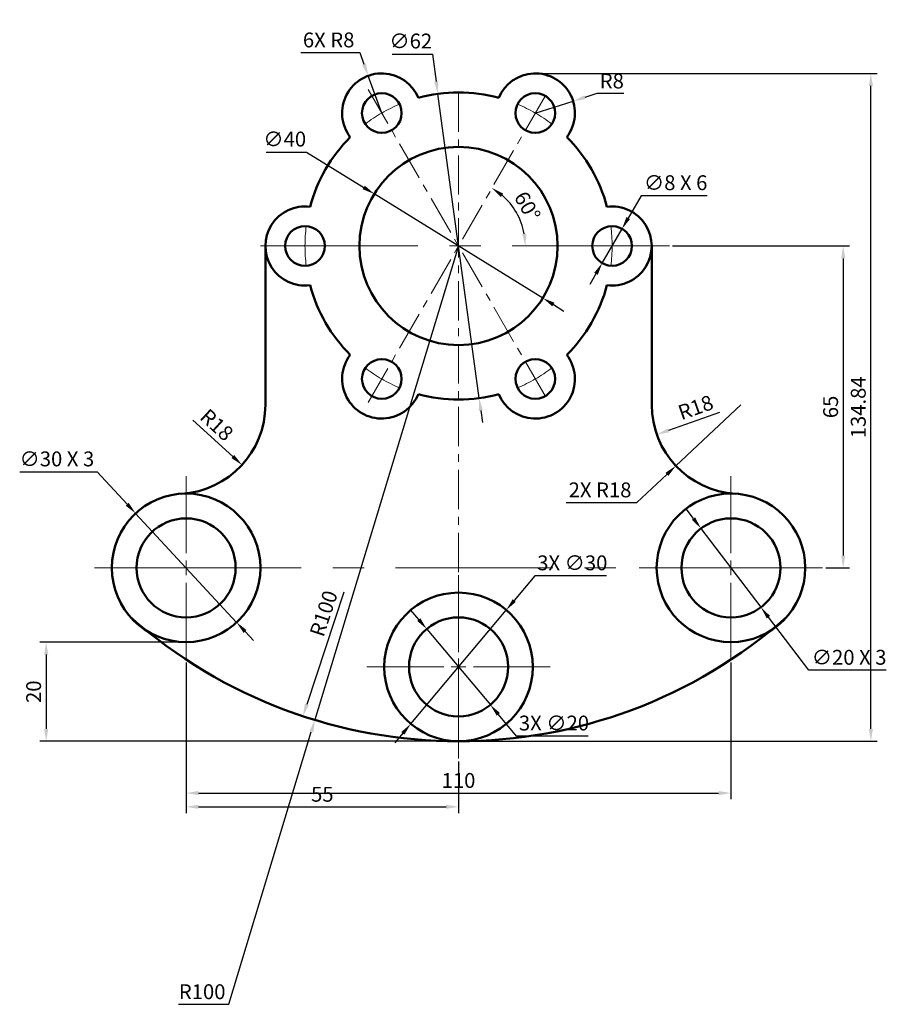
# Model space of a CAD drawing. Units: millimetres. Extents: x 7601 to 7776, y 4114 to 4313.
import ezdxf

# ---------------------------------------------------------------- set-up
doc = ezdxf.new("R2010")
doc.units = ezdxf.units.MM
doc.linetypes.add('CENTER', pattern=[50.8, 31.75, -6.35, 6.35, -6.35])
for name, color, linetype, lineweight in [('M-CNTR', 1, 'CENTER', 18), ('M-DIMS', 2, 'Continuous', 25), ('M-OUTL', 7, 'Continuous', 50)]:
    doc.layers.add(name, color=color, linetype=linetype, lineweight=lineweight)
doc.styles.get("Standard").update_dxf_attribs({"font": 'arial.ttf'})
doc.dimstyles.new('ISO-25', dxfattribs={"dimtxt": 3, "dimasz": 2.5, "dimexe": 1.25, "dimexo": 0.625, "dimtad": 1, "dimtoh": 1, "dimdec": 0, "dimtxsty": 'Standard', "dimcen": 2.5, "dimadec": 0, "dimazin": 0, "dimtfac": 1, "dimtdec": 0, "dimtmove": 0, "dimatfit": 3, "dimfxl": 1, "dimarcsym": 0})

# ---------------------------------------------------------------- blocks, each defined once
blk = doc.blocks.new('*U1')
at = {"layer": 'M-CNTR', "color": 0, "transparency": 16777216}
for p, q in [((0, 3), (0, 18.5)), ((-18.5, 0), (-3, 0)), ((3, 0), (18.5, 0)), ((0, -18.5), (0, -3))]:
    blk.add_line(p, q, dxfattribs=at)
at = {"layer": 'M-CNTR', "color": 0, "linetype": 'Continuous', "transparency": 16777216}
for p, q in [((-1.5, 0), (1.5, 0)), ((0, -1.5), (0, 1.5))]:
    blk.add_line(p, q, dxfattribs=at)
blk = doc.blocks.new('*U2')
at = {"layer": 'M-CNTR', "color": 0, "transparency": 16777216}
for p, q in [((0, 3), (0, 18.5)), ((-18.5, 0), (-3, 0)), ((3, 0), (18.5, 0)), ((0, -18.5), (0, -3))]:
    blk.add_line(p, q, dxfattribs=at)
at = {"layer": 'M-CNTR', "color": 0, "linetype": 'Continuous', "transparency": 16777216}
for p, q in [((-1.5, 0), (1.5, 0)), ((0, -1.5), (0, 1.5))]:
    blk.add_line(p, q, dxfattribs=at)
blk = doc.blocks.new('*U3')
at = {"layer": 'M-CNTR', "color": 0, "transparency": 16777216}
for p, q in [((0, 3), (0, 18.5)), ((-18.5, 0), (-3, 0)), ((3, 0), (18.5, 0)), ((0, -18.5), (0, -3))]:
    blk.add_line(p, q, dxfattribs=at)
at = {"layer": 'M-CNTR', "color": 0, "linetype": 'Continuous', "transparency": 16777216}
for p, q in [((-1.5, 0), (1.5, 0)), ((0, -1.5), (0, 1.5))]:
    blk.add_line(p, q, dxfattribs=at)
blk = doc.blocks.new('*D4')
at = {"layer": 'Defpoints', "color": 0, "transparency": 16777216}
for p in [(7634.97, 4183.77), (7744.97, 4183.77), (7744.97, 4156.8)]:
    blk.add_point(p, dxfattribs=at)
at = {"layer": 'M-DIMS', "color": 0, "lineweight": -2, "transparency": 16777216}
for p, q in [((7634.97, 4183.15), (7634.97, 4155.55)), ((7744.97, 4183.15), (7744.97, 4155.55)), ((7637.47, 4156.8), (7742.47, 4156.8))]:
    blk.add_line(p, q, dxfattribs=at)
at = {"layer": 'M-DIMS', "color": 0, "transparency": 16777216}
for points in [[(7637.47, 4157.22), (7637.47, 4156.39), (7634.97, 4156.8)], [(7742.47, 4157.22), (7742.47, 4156.39), (7744.97, 4156.8)]]:
    blk.add_solid(points, dxfattribs=at)
at = {"layer": 'M-DIMS', "color": 0, "transparency": 16777216, "insert": (7689.97, 4158.96), "char_height": 3, "attachment_point": 5}
blk.add_mtext('110', dxfattribs=at)
blk = doc.blocks.new('*D7')
at = {"layer": 'Defpoints', "color": 0, "transparency": 16777216}
for p in [(7624.78, 4213.27), (7645.17, 4191.27)]:
    blk.add_point(p, dxfattribs=at)
at = {"layer": 'M-DIMS', "color": 0, "lineweight": -2, "transparency": 16777216}
for p, q in [((7601.37, 4221.65), (7617.01, 4221.65)), ((7617.01, 4221.65), (7623.08, 4215.11)), ((7645.17, 4191.27), (7624.78, 4213.27)), ((7646.87, 4189.44), (7648.57, 4187.6))]:
    blk.add_line(p, q, dxfattribs=at)
at = {"layer": 'M-DIMS', "color": 0, "transparency": 16777216}
for points in [[(7623.38, 4215.39), (7622.77, 4214.83), (7624.78, 4213.27)], [(7647.17, 4189.72), (7646.56, 4189.15), (7645.17, 4191.27)]]:
    blk.add_solid(points, dxfattribs=at)
at = {"layer": 'M-DIMS', "color": 0, "transparency": 16777216, "insert": (7608.88, 4223.89), "char_height": 3, "attachment_point": 5}
blk.add_mtext('∅30 X 3', dxfattribs=at)
blk = doc.blocks.new('*D8')
at = {"layer": 'Defpoints', "color": 0, "transparency": 16777216}
for p in [(7738.92, 4210.23), (7751.02, 4194.31)]:
    blk.add_point(p, dxfattribs=at)
at = {"layer": 'M-DIMS', "color": 0, "lineweight": -2, "transparency": 16777216}
for p, q in [((7737.41, 4212.22), (7735.9, 4214.21)), ((7738.92, 4210.23), (7751.02, 4194.31)), ((7760.7, 4181.59), (7752.54, 4192.32)), ((7776.34, 4181.59), (7760.7, 4181.59))]:
    blk.add_line(p, q, dxfattribs=at)
at = {"layer": 'M-DIMS', "color": 0, "transparency": 16777216}
for points in [[(7737.74, 4212.48), (7737.08, 4211.97), (7738.92, 4210.23)], [(7752.87, 4192.57), (7752.21, 4192.07), (7751.02, 4194.31)]]:
    blk.add_solid(points, dxfattribs=at)
at = {"layer": 'M-DIMS', "color": 0, "transparency": 16777216, "insert": (7768.83, 4183.83), "char_height": 3, "attachment_point": 5}
blk.add_mtext('∅20 X 3', dxfattribs=at)
blk = doc.blocks.new('*D5')
at = {"layer": 'Defpoints', "color": 0, "transparency": 16777216}
for p in [(7689.97, 4267.27), (7658.56, 4172.34)]:
    blk.add_point(p, dxfattribs=at)
at = {"layer": 'M-DIMS', "color": 0, "lineweight": -2, "transparency": 16777216}
blk.add_line((7666.84, 4197.37), (7659.34, 4174.71), dxfattribs=at)
at = {"layer": 'M-DIMS', "color": 0, "transparency": 16777216}
blk.add_solid([(7658.95, 4174.84), (7659.74, 4174.58), (7658.56, 4172.34)], dxfattribs=at)
at = {"layer": 'M-DIMS', "color": 0, "transparency": 16777216, "insert": (7663.11, 4192.95), "char_height": 3, "attachment_point": 5, "rotation": 71.6889}
blk.add_mtext('R100', dxfattribs=at)
blk = doc.blocks.new('*D6')
at = {"layer": 'Defpoints', "color": 0, "transparency": 16777216}
for p in [(7632.97, 4235.21), (7646.26, 4223.06)]:
    blk.add_point(p, dxfattribs=at)
at = {"layer": 'M-DIMS', "color": 0, "lineweight": -2, "transparency": 16777216}
blk.add_line((7636.35, 4232.12), (7644.41, 4224.75), dxfattribs=at)
at = {"layer": 'M-DIMS', "color": 0, "transparency": 16777216}
blk.add_solid([(7644.69, 4225.06), (7644.13, 4224.44), (7646.26, 4223.06)], dxfattribs=at)
at = {"layer": 'M-DIMS', "color": 0, "transparency": 16777216, "insert": (7640.91, 4230.87), "char_height": 3, "attachment_point": 5, "rotation": 317.5585}
blk.add_mtext('R18', dxfattribs=at)
blk = doc.blocks.new('*D9')
at = {"layer": 'Defpoints', "color": 0, "transparency": 16777216}
for p in [(7713.1, 4296.53), (7705.47, 4294.12)]:
    blk.add_point(p, dxfattribs=at)
at = {"layer": 'M-DIMS', "color": 0, "lineweight": -2, "transparency": 16777216}
for p, q in [((7705.47, 4294.12), (7713.1, 4296.53)), ((7717.87, 4298.04), (7715.49, 4297.28)), ((7723.34, 4298.04), (7717.87, 4298.04))]:
    blk.add_line(p, q, dxfattribs=at)
at = {"layer": 'M-DIMS', "color": 0, "transparency": 16777216}
blk.add_solid([(7715.36, 4297.68), (7715.61, 4296.89), (7713.1, 4296.53)], dxfattribs=at)
at = {"layer": 'M-DIMS', "color": 0, "transparency": 16777216, "insert": (7720.92, 4300.19), "char_height": 3, "attachment_point": 5}
blk.add_mtext('R8', dxfattribs=at)
blk = doc.blocks.new('*D10')
at = {"layer": 'Defpoints', "color": 0, "transparency": 16777216}
for p in [(7746.97, 4235.21), (7730.01, 4229.2)]:
    blk.add_point(p, dxfattribs=at)
at = {"layer": 'M-DIMS', "color": 0, "lineweight": -2, "transparency": 16777216}
blk.add_line((7742.66, 4233.68), (7732.36, 4230.04), dxfattribs=at)
at = {"layer": 'M-DIMS', "color": 0, "transparency": 16777216}
blk.add_solid([(7732.22, 4230.43), (7732.5, 4229.64), (7730.01, 4229.2)], dxfattribs=at)
at = {"layer": 'M-DIMS', "color": 0, "transparency": 16777216, "insert": (7737.97, 4234.31), "char_height": 3, "attachment_point": 5, "rotation": 19.5016}
blk.add_mtext('R18', dxfattribs=at)
blk = doc.blocks.new('*D11')
at = {"layer": 'Defpoints', "color": 0, "transparency": 16777216}
for p in [(7685.81, 4297.99), (7694.13, 4236.55)]:
    blk.add_point(p, dxfattribs=at)
at = {"layer": 'M-DIMS', "color": 0, "lineweight": -2, "transparency": 16777216}
for p, q in [((7676.57, 4306.03), (7684.72, 4306.03)), ((7684.72, 4306.03), (7685.48, 4300.47)), ((7694.13, 4236.55), (7685.81, 4297.99)), ((7694.47, 4234.08), (7694.81, 4231.6))]:
    blk.add_line(p, q, dxfattribs=at)
at = {"layer": 'M-DIMS', "color": 0, "transparency": 16777216}
for points in [[(7685.89, 4300.53), (7685.06, 4300.41), (7685.81, 4297.99)], [(7694.88, 4234.13), (7694.06, 4234.02), (7694.13, 4236.55)]]:
    blk.add_solid(points, dxfattribs=at)
at = {"layer": 'M-DIMS', "color": 0, "transparency": 16777216, "insert": (7680.33, 4308.27), "char_height": 3, "attachment_point": 5}
blk.add_mtext('∅62', dxfattribs=at)
blk = doc.blocks.new('*D12')
at = {"layer": 'Defpoints', "color": 0, "transparency": 16777216}
for p in [(7672.96, 4277.78), (7706.99, 4256.76)]:
    blk.add_point(p, dxfattribs=at)
at = {"layer": 'M-DIMS', "color": 0, "lineweight": -2, "transparency": 16777216}
for p, q in [((7651.1, 4286.23), (7659.28, 4286.23)), ((7659.28, 4286.23), (7670.83, 4279.09)), ((7706.99, 4256.76), (7672.96, 4277.78)), ((7709.12, 4255.45), (7711.24, 4254.14))]:
    blk.add_line(p, q, dxfattribs=at)
at = {"layer": 'M-DIMS', "color": 0, "transparency": 16777216}
for points in [[(7671.05, 4279.45), (7670.61, 4278.74), (7672.96, 4277.78)], [(7709.34, 4255.81), (7708.9, 4255.1), (7706.99, 4256.76)]]:
    blk.add_solid(points, dxfattribs=at)
at = {"layer": 'M-DIMS', "color": 0, "transparency": 16777216, "insert": (7654.88, 4288.47), "char_height": 3, "attachment_point": 5}
blk.add_mtext('∅40', dxfattribs=at)
blk = doc.blocks.new('*D13')
at = {"layer": 'Defpoints', "color": 0, "transparency": 16777216}
for p in [(7722.98, 4270.73), (7718.97, 4263.81)]:
    blk.add_point(p, dxfattribs=at)
at = {"layer": 'M-DIMS', "color": 0, "lineweight": -2, "transparency": 16777216}
for p, q in [((7726.85, 4277.42), (7724.23, 4272.9)), ((7740.15, 4277.42), (7726.85, 4277.42)), ((7718.97, 4263.81), (7722.98, 4270.73)), ((7717.72, 4261.65), (7716.46, 4259.48))]:
    blk.add_line(p, q, dxfattribs=at)
at = {"layer": 'M-DIMS', "color": 0, "transparency": 16777216}
for points in [[(7723.87, 4273.11), (7724.59, 4272.69), (7722.98, 4270.73)], [(7717.36, 4261.86), (7718.08, 4261.44), (7718.97, 4263.81)]]:
    blk.add_solid(points, dxfattribs=at)
at = {"layer": 'M-DIMS', "color": 0, "transparency": 16777216, "insert": (7733.81, 4279.66), "char_height": 3, "attachment_point": 5}
blk.add_mtext('∅8 X 6', dxfattribs=at)
blk = doc.blocks.new('*D14')
at = {"layer": 'Defpoints', "color": 0, "transparency": 16777216}
for p in [(7732.57, 4267.27), (7763.47, 4202.27), (7767.64, 4202.27)]:
    blk.add_point(p, dxfattribs=at)
at = {"layer": 'M-DIMS', "color": 0, "lineweight": -2, "transparency": 16777216}
for p, q in [((7733.2, 4267.27), (7768.89, 4267.27)), ((7767.64, 4264.77), (7767.64, 4204.77)), ((7764.1, 4202.27), (7768.89, 4202.27))]:
    blk.add_line(p, q, dxfattribs=at)
at = {"layer": 'M-DIMS', "color": 0, "transparency": 16777216}
for points in [[(7767.22, 4264.77), (7768.05, 4264.77), (7767.64, 4267.27)], [(7767.22, 4204.77), (7768.05, 4204.77), (7767.64, 4202.27)]]:
    blk.add_solid(points, dxfattribs=at)
at = {"layer": 'M-DIMS', "color": 0, "transparency": 16777216, "insert": (7765.48, 4234.77), "char_height": 3, "attachment_point": 5, "rotation": 90}
blk.add_mtext('65', dxfattribs=at)
blk = doc.blocks.new('*D15')
at = {"layer": 'Defpoints', "color": 0, "transparency": 16777216}
for p in [(7708.22, 4298.88), (7702.66, 4271.89), (7647.37, 4267.27), (7732.57, 4267.27), (7671.72, 4235.66)]:
    blk.add_point(p, dxfattribs=at)
at = {"layer": 'M-DIMS', "color": 0, "lineweight": -2, "transparency": 16777216}
blk.add_arc((7689.97, 4267.27), 13.5, 10.6241, 49.3759, dxfattribs=at)
at = {"layer": 'M-DIMS', "color": 0, "transparency": 16777216}
for points in [[(7698.52, 4277.18), (7699, 4277.86), (7696.72, 4278.97)], [(7703.66, 4269.8), (7702.83, 4269.72), (7703.47, 4267.27)]]:
    blk.add_solid(points, dxfattribs=at)
at = {"layer": 'M-DIMS', "color": 0, "transparency": 16777216, "insert": (7703.53, 4275.1), "char_height": 3, "attachment_point": 5, "rotation": 300}
blk.add_mtext('60°', dxfattribs=at)
blk = doc.blocks.new('FLANGE-LUG-D8')
blk.add_circle((0, 0), 4)
blk.add_arc((0, 0), 8, 262.5863, 97.4137)
blk = doc.blocks.new('PIVOT-EYE-D30-D20')
for radius in [15, 10]:
    blk.add_circle((0, 0), radius)
blk = doc.blocks.new('*D18')
at = {"layer": 'Defpoints', "color": 0, "transparency": 16777216}
for p in [(7634.97, 4187.27), (7606.72, 4167.27), (7689.97, 4167.27)]:
    blk.add_point(p, dxfattribs=at)
at = {"layer": 'M-DIMS', "color": 0, "lineweight": -2, "transparency": 16777216}
for p, q in [((7634.35, 4187.27), (7605.47, 4187.27)), ((7606.72, 4184.77), (7606.72, 4169.77)), ((7689.35, 4167.27), (7605.47, 4167.27))]:
    blk.add_line(p, q, dxfattribs=at)
at = {"layer": 'M-DIMS', "color": 0, "transparency": 16777216}
for points in [[(7606.31, 4184.77), (7607.14, 4184.77), (7606.72, 4187.27)], [(7606.31, 4169.77), (7607.14, 4169.77), (7606.72, 4167.27)]]:
    blk.add_solid(points, dxfattribs=at)
at = {"layer": 'M-DIMS', "color": 0, "transparency": 16777216, "insert": (7604.57, 4177.27), "char_height": 3, "attachment_point": 5, "rotation": 90}
blk.add_mtext('20', dxfattribs=at)
blk = doc.blocks.new('*D19')
at = {"layer": 'Defpoints', "color": 0, "transparency": 16777216}
for p in [(7705.13, 4302.11), (7773.22, 4302.11), (7689.97, 4167.27)]:
    blk.add_point(p, dxfattribs=at)
at = {"layer": 'M-DIMS', "color": 0, "lineweight": -2, "transparency": 16777216}
for p, q in [((7705.75, 4302.11), (7774.47, 4302.11)), ((7773.22, 4169.77), (7773.22, 4299.61)), ((7690.6, 4167.27), (7774.47, 4167.27))]:
    blk.add_line(p, q, dxfattribs=at)
at = {"layer": 'M-DIMS', "color": 0, "transparency": 16777216}
for points in [[(7772.81, 4299.61), (7773.64, 4299.61), (7773.22, 4302.11)], [(7772.81, 4169.77), (7773.64, 4169.77), (7773.22, 4167.27)]]:
    blk.add_solid(points, dxfattribs=at)
at = {"layer": 'M-DIMS', "color": 0, "transparency": 16777216, "insert": (7771.07, 4234.69), "char_height": 3, "attachment_point": 5, "rotation": 90}
blk.add_mtext('134.84', dxfattribs=at)
blk = doc.blocks.new('*D20')
at = {"layer": 'Defpoints', "color": 0, "transparency": 16777216}
for p in [(7634.97, 4183.77), (7689.97, 4163.77), (7689.97, 4154.02)]:
    blk.add_point(p, dxfattribs=at)
at = {"layer": 'M-DIMS', "color": 0, "lineweight": -2, "transparency": 16777216}
for p, q in [((7634.97, 4183.15), (7634.97, 4152.77)), ((7689.97, 4163.15), (7689.97, 4152.77)), ((7637.47, 4154.02), (7687.47, 4154.02))]:
    blk.add_line(p, q, dxfattribs=at)
at = {"layer": 'M-DIMS', "color": 0, "transparency": 16777216}
for points in [[(7637.47, 4154.44), (7637.47, 4153.61), (7634.97, 4154.02)], [(7687.47, 4154.44), (7687.47, 4153.61), (7689.97, 4154.02)]]:
    blk.add_solid(points, dxfattribs=at)
at = {"layer": 'M-DIMS', "color": 0, "transparency": 16777216, "insert": (7662.47, 4156.17), "char_height": 3, "attachment_point": 5}
blk.add_mtext('55', dxfattribs=at)
blk = doc.blocks.new('*D21')
at = {"layer": 'Defpoints', "color": 0, "transparency": 16777216}
for p in [(7671.74, 4301.64), (7674.47, 4294.12)]:
    blk.add_point(p, dxfattribs=at)
at = {"layer": 'M-DIMS', "color": 0, "lineweight": -2, "transparency": 16777216}
for p, q in [((7658.1, 4306.34), (7670.03, 4306.34)), ((7670.03, 4306.34), (7670.88, 4303.99)), ((7674.47, 4294.12), (7671.74, 4301.64))]:
    blk.add_line(p, q, dxfattribs=at)
at = {"layer": 'M-DIMS', "color": 0, "transparency": 16777216}
blk.add_solid([(7671.27, 4304.13), (7670.49, 4303.84), (7671.74, 4301.64)], dxfattribs=at)
at = {"layer": 'M-DIMS', "color": 0, "transparency": 16777216, "insert": (7663.75, 4308.49), "char_height": 3, "attachment_point": 5}
blk.add_mtext('6X R8', dxfattribs=at)
blk = doc.blocks.new('*D22')
at = {"layer": 'Defpoints', "color": 0, "transparency": 16777216}
for p in [(7746.97, 4235.21), (7733.86, 4222.88)]:
    blk.add_point(p, dxfattribs=at)
at = {"layer": 'M-DIMS', "color": 0, "lineweight": -2, "transparency": 16777216}
for p, q in [((7746.97, 4235.21), (7733.86, 4222.88)), ((7726, 4215.47), (7732.04, 4221.16)), ((7711.7, 4215.47), (7726, 4215.47))]:
    blk.add_line(p, q, dxfattribs=at)
at = {"layer": 'M-DIMS', "color": 0, "transparency": 16777216}
blk.add_solid([(7731.76, 4221.47), (7732.33, 4220.86), (7733.86, 4222.88)], dxfattribs=at)
at = {"layer": 'M-DIMS', "color": 0, "transparency": 16777216, "insert": (7718.54, 4217.63), "char_height": 3, "attachment_point": 5}
blk.add_mtext('2X R18', dxfattribs=at)
blk = doc.blocks.new('*D23')
at = {"layer": 'Defpoints', "color": 0, "transparency": 16777216}
for p in [(7699.61, 4193.76), (7680.33, 4170.78)]:
    blk.add_point(p, dxfattribs=at)
at = {"layer": 'M-DIMS', "color": 0, "lineweight": -2, "transparency": 16777216}
for p, q in [((7705.4, 4200.66), (7701.22, 4195.68)), ((7719.86, 4200.66), (7705.4, 4200.66)), ((7680.33, 4170.78), (7699.61, 4193.76)), ((7678.72, 4168.87), (7677.12, 4166.95))]:
    blk.add_line(p, q, dxfattribs=at)
at = {"layer": 'M-DIMS', "color": 0, "transparency": 16777216}
for points in [[(7700.9, 4195.95), (7701.54, 4195.41), (7699.61, 4193.76)], [(7678.41, 4169.13), (7679.04, 4168.6), (7680.33, 4170.78)]]:
    blk.add_solid(points, dxfattribs=at)
at = {"layer": 'M-DIMS', "color": 0, "transparency": 16777216, "insert": (7712.94, 4202.9), "char_height": 3, "attachment_point": 5}
blk.add_mtext('3X ∅30', dxfattribs=at)
blk = doc.blocks.new('*D24')
at = {"layer": 'Defpoints', "color": 0, "transparency": 16777216}
for p in [(7683.54, 4189.93), (7696.4, 4174.61)]:
    blk.add_point(p, dxfattribs=at)
at = {"layer": 'M-DIMS', "color": 0, "lineweight": -2, "transparency": 16777216}
for p, q in [((7681.94, 4191.85), (7680.33, 4193.76)), ((7683.54, 4189.93), (7696.4, 4174.61)), ((7701.69, 4168.31), (7698.01, 4172.7)), ((7716.15, 4168.31), (7701.69, 4168.31))]:
    blk.add_line(p, q, dxfattribs=at)
at = {"layer": 'M-DIMS', "color": 0, "transparency": 16777216}
for points in [[(7682.26, 4192.12), (7681.62, 4191.58), (7683.54, 4189.93)], [(7698.33, 4172.97), (7697.69, 4172.43), (7696.4, 4174.61)]]:
    blk.add_solid(points, dxfattribs=at)
at = {"layer": 'M-DIMS', "color": 0, "transparency": 16777216, "insert": (7709.24, 4170.55), "char_height": 3, "attachment_point": 5}
blk.add_mtext('3X ∅20', dxfattribs=at)
blk = doc.blocks.new('*D25')
at = {"layer": 'Defpoints', "color": 0, "transparency": 16777216}
for p in [(7689.97, 4267.27), (7660.98, 4171.57)]:
    blk.add_point(p, dxfattribs=at)
at = {"layer": 'M-DIMS', "color": 0, "lineweight": -2, "transparency": 16777216}
for p, q in [((7689.97, 4267.27), (7660.98, 4171.57)), ((7643.58, 4114.15), (7660.25, 4169.18)), ((7633.46, 4114.15), (7643.58, 4114.15))]:
    blk.add_line(p, q, dxfattribs=at)
at = {"layer": 'M-DIMS', "color": 0, "transparency": 16777216}
blk.add_solid([(7659.85, 4169.3), (7660.65, 4169.06), (7660.98, 4171.57)], dxfattribs=at)
at = {"layer": 'M-DIMS', "color": 0, "transparency": 16777216, "insert": (7638.21, 4116.3), "char_height": 3, "attachment_point": 5}
blk.add_mtext('R100', dxfattribs=at)

msp = doc.modelspace()

# ---------------------------------------------------------------- linework, layer by layer
at = {"layer": 'M-CNTR', "ltscale": 0.25}
for p, q in [((7671.722, 4235.661), (7708.224, 4298.885)), ((7671.722, 4298.885), (7708.224, 4235.661)), ((7689.973, 4298.273), (7689.973, 4167.273)), ((7689.973, 4298.273), (7689.973, 4167.273))]:
    msp.add_line(p, q, dxfattribs=at)
at = {"layer": 'M-CNTR'}
for p, q in [((7732.572, 4267.273), (7647.374, 4267.273)), ((7759.828, 4202.273), (7620.119, 4202.273))]:
    msp.add_line(p, q, dxfattribs=at)
for start, end in [(112.60186, 127.39814), (52.60186, 67.39814), (172.60186, 187.39814), (352.60186, 7.39814), (232.60186, 247.39814), (292.60186, 307.39814)]:
    msp.add_arc((7689.973, 4267.273), 31, start, end, dxfattribs=at)
at = {"layer": 'M-OUTL'}
for p, q in [((7650.973, 4267.273), (7650.973, 4235.212)), ((7728.973, 4267.273), (7728.973, 4235.212))]:
    msp.add_line(p, q, dxfattribs=at)
msp.add_circle((7689.973, 4267.273), 20, dxfattribs=at)
for centre, radius, start, end in [((7689.973, 4267.273), 31, 74.82735, 105.17265), ((7689.973, 4267.273), 31, 134.82735, 165.17265), ((7689.973, 4267.273), 31, 14.82735, 45.17265), ((7689.973, 4267.273), 31, 194.82735, 225.17265), ((7689.973, 4267.273), 31, 314.82735, 345.17265), ((7689.973, 4267.273), 31, 254.82735, 285.17265), ((7632.973, 4235.212), 18, 273.4746, 0), ((7746.973, 4235.212), 18, 180, 266.5254), ((7689.973, 4267.273), 100, 228.46317, 311.53683)]:
    msp.add_arc(centre, radius, start, end, dxfattribs=at)

# ---------------------------------------------------------------- block references
at = {"layer": 'M-CNTR'}
for name, p in [('*U3', (7634.973, 4202.273)), ('*U2', (7744.973, 4202.273)), ('*U1', (7689.973, 4182.273))]:
    msp.add_blockref(name, p, dxfattribs=at)
at = {"layer": 'M-OUTL'}
for p, rotation in [((7674.473, 4294.119), 119.9999999998415), ((7705.473, 4294.119), 60.00000000001975), ((7658.973, 4267.273), 180), ((7674.473, 4240.426), 240.0000000000073), ((7705.473, 4240.426), 299.9999999990406)]:
    msp.add_blockref('FLANGE-LUG-D8', p, dxfattribs=dict(at, rotation=rotation))
for name, p in [('FLANGE-LUG-D8', (7720.973, 4267.273)), ('PIVOT-EYE-D30-D20', (7634.973, 4202.273)), ('PIVOT-EYE-D30-D20', (7744.973, 4202.273)), ('PIVOT-EYE-D30-D20', (7689.973, 4182.273))]:
    msp.add_blockref(name, p, dxfattribs=at)

# ---------------------------------------------------------------- dimensions: what is measured, and where the dimension line sits
at = {"layer": 'M-DIMS'}
dim = msp.add_radius_dim(center=(7674.473, 4294.119), mpoint=(7671.737, 4301.637), text='6X <>', dimstyle='ISO-25', override={"dimdec": 0, "dimlfac": 1, "dimrnd": 0, "dimzin": 0, "dimdsep": 46, "dimlunit": 2}, dxfattribs=at)
dim.commit()
dim.dimension.update_dxf_attribs({"geometry": '*D21', "text_midpoint": (7663.749, 4308.492)})
for p1, p2, picture, middle in [((7694.134, 4236.553), (7685.812, 4297.992), '*D11', (7680.333, 4306.028)), ((7706.99, 4256.764), (7672.956, 4277.781), '*D12', (7654.876, 4286.229))]:
    dim = msp.add_diameter_dim_2p(p1=p1, p2=p2, dimstyle='ISO-25', override={"dimclrd": 0, "dimclre": 0, "dimclrt": 0}, dxfattribs=at)
    dim.commit()
    dim.dimension.update_dxf_attribs({"geometry": picture, "text_midpoint": middle, "dimtype": 163})
for base, p1, p2, override, picture, middle in [((7773.223, 4302.112), (7689.973, 4167.273), (7705.128, 4302.112), {"dimdec": 2, "dimlfac": 1, "dimrnd": 0, "dimzin": 0, "dimdsep": 46, "dimlunit": 2}, '*D19', (7771.065, 4234.692)), ((7767.636, 4202.273), (7732.572, 4267.273), (7763.473, 4202.273), {"dimclrd": 0, "dimclre": 0, "dimclrt": 0}, '*D14', (7765.479, 4234.773)), ((7606.723, 4167.273), (7634.973, 4187.273), (7689.973, 4167.273), {"dimdec": 0, "dimlfac": 1, "dimrnd": 0, "dimzin": 0, "dimdsep": 46, "dimlunit": 2}, '*D18', (7604.566, 4177.273))]:
    dim = msp.add_linear_dim(base=base, p1=p1, p2=p2, angle=90, dimstyle='ISO-25', override=override, dxfattribs=at)
    dim.commit()
    dim.dimension.update_dxf_attribs({"geometry": picture, "text_midpoint": middle})
dim = msp.add_radius_dim(center=(7705.473, 4294.119), mpoint=(7713.101, 4296.53), dimstyle='ISO-25', override={"dimclrd": 0, "dimclre": 0, "dimclrt": 0}, dxfattribs=at)
dim.commit()
dim.dimension.update_dxf_attribs({"geometry": '*D9', "text_midpoint": (7720.916, 4300.193)})
dim = msp.add_angular_dim_2l(base=(7702.661, 4271.891), line1=((7671.722, 4235.661), (7708.224, 4298.885)), line2=((7732.572, 4267.273), (7647.374, 4267.273)), dimstyle='ISO-25', override={"dimclrd": 0, "dimclre": 0, "dimclrt": 0}, dxfattribs=at)
dim.commit()
dim.dimension.update_dxf_attribs({"geometry": '*D15', "text_midpoint": (7703.534, 4275.102)})
for p1, p2, text, override, picture, middle in [((7718.969, 4263.811), (7722.977, 4270.734), '<> X 6', {"dimclrd": 0, "dimclre": 0, "dimclrt": 0}, '*D13', (7733.813, 4277.416)), ((7645.169, 4191.271), (7624.777, 4213.275), '<> X 3', {"dimclrd": 0, "dimclre": 0, "dimclrt": 0}, '*D7', (7608.879, 4221.653)), ((7738.922, 4210.234), (7751.024, 4194.311), '<> X 3', {"dimclrd": 0, "dimclre": 0, "dimclrt": 0}, '*D8', (7768.828, 4181.588)), ((7680.332, 4170.782), (7699.615, 4193.764), '3X <>', {"dimdec": 0, "dimlfac": 1, "dimrnd": 0, "dimzin": 0, "dimdsep": 46, "dimlunit": 2}, '*D23', (7712.942, 4200.658)), ((7683.545, 4189.933), (7696.401, 4174.613), '3X <>', {"dimdec": 0, "dimlfac": 1, "dimrnd": 0, "dimzin": 0, "dimdsep": 46, "dimlunit": 2}, '*D24', (7709.235, 4168.307))]:
    dim = msp.add_diameter_dim_2p(p1=p1, p2=p2, text=text, dimstyle='ISO-25', override=override, dxfattribs=at)
    dim.commit()
    dim.dimension.update_dxf_attribs({"geometry": picture, "text_midpoint": middle, "dimtype": 163})
for center, mpoint, override, picture, middle in [((7689.973, 4267.273), (7660.976, 4171.569), {"dimdec": 0, "dimlfac": 1, "dimrnd": 0, "dimzin": 0, "dimdsep": 46, "dimlunit": 2}, '*D25', (7638.208, 4114.147)), ((7689.973, 4267.273), (7658.556, 4172.336), {"dimclrd": 0, "dimclre": 0, "dimclrt": 0}, '*D5', (7665.153, 4192.273)), ((7746.973, 4235.212), (7730.006, 4229.203), {"dimclrd": 0, "dimclre": 0, "dimclrt": 0}, '*D10', (7738.69, 4232.278)), ((7632.973, 4235.212), (7646.256, 4223.065), {"dimclrd": 0, "dimclre": 0, "dimclrt": 0}, '*D6', (7639.458, 4229.282))]:
    dim = msp.add_radius_dim(center=center, mpoint=mpoint, dimstyle='ISO-25', override=override, dxfattribs=at)
    dim.commit()
    dim.dimension.update_dxf_attribs({"geometry": picture, "text_midpoint": middle, "dimtype": 164})
dim = msp.add_radius_dim(center=(7746.973, 4235.212), mpoint=(7733.865, 4222.876), text='2X <>', dimstyle='ISO-25', override={"dimdec": 0, "dimlfac": 1, "dimrnd": 0, "dimzin": 0, "dimdsep": 46, "dimlunit": 2}, dxfattribs=at)
dim.commit()
dim.dimension.update_dxf_attribs({"geometry": '*D22', "text_midpoint": (7718.539, 4215.474), "dimtype": 164})
for base, p2, override, picture, middle in [((7744.973, 4156.802), (7744.973, 4183.773), {"dimclrd": 0, "dimclre": 0, "dimclrt": 0}, '*D4', (7689.973, 4158.959)), ((7689.973, 4154.023), (7689.973, 4163.773), {"dimdec": 0, "dimlfac": 1, "dimrnd": 0, "dimzin": 0, "dimdsep": 46, "dimlunit": 2}, '*D20', (7662.473, 4156.173))]:
    dim = msp.add_linear_dim(base=base, p1=(7634.973, 4183.773), p2=p2, dimstyle='ISO-25', override=override, dxfattribs=at)
    dim.commit()
    dim.dimension.update_dxf_attribs({"geometry": picture, "text_midpoint": middle})

doc.saveas('drawing.dxf')
